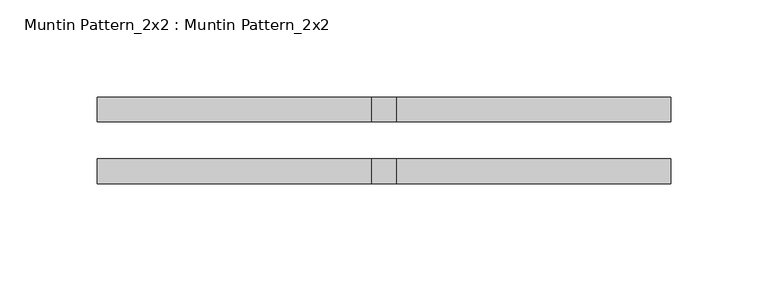
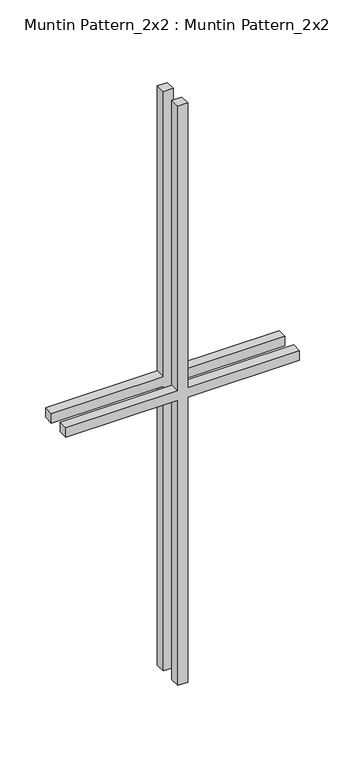
"""IFC4 building model written with IfcOpenShell, lengths in millimetres: proxy geometry, Muntin Pattern_2x2 : Muntin Pattern_2x2."""

from ifc_helpers import new_model, si_unit, frame, origin, place, context, project, spatial, polyline, outline, extrude, source, transform, mapped, element, save


def muntin_pattern_2x2_muntin_pattern_2x2_b3fe6957(model_context):
    return source(origin(), model_context, "Body", "SweptSolid", [
        extrude(outline(polyline([(393.7, -6.35), (393.7, -147.6375), (381.0, -147.6375), (381.0, -6.35), (0.0, -6.35), (0.0, 6.35), (381.0, 6.35), (381.0, 147.6375), (393.7, 147.6375), (393.7, 6.35), (774.7, 6.35), (774.7, -6.35), (393.7, -6.35)])), frame((0.0, 9.525, 0.0), z_axis=(0.0, 1.0, 0.0), x_axis=(0.0, 0.0, 1.0)), (0.0, 0.0, 1.0), 12.7),
        extrude(outline(polyline([(393.7, -6.35), (393.7, -147.6375), (381.0, -147.6375), (381.0, -6.35), (0.0, -6.35), (0.0, 6.35), (381.0, 6.35), (381.0, 147.6375), (393.7, 147.6375), (393.7, 6.35), (774.7, 6.35), (774.7, -6.35), (393.7, -6.35)])), frame((0.0, -22.225, 0.0), z_axis=(0.0, 1.0, 0.0), x_axis=(0.0, 0.0, 1.0)), (0.0, 0.0, 1.0), 12.7),
    ])


if __name__ == "__main__":
    model = new_model("IFC4")
    model_context = context("Model", 3, world=origin())
    ifc_project = project(units=[si_unit("LENGTHUNIT", "METRE", prefix="MILLI")], contexts=[model_context])
    site = spatial("IfcSite", under=ifc_project)
    building = spatial("IfcBuilding", under=site)
    placement = place(None, origin())
    muntin_pattern_2x2_muntin_pattern_2x2_shape = muntin_pattern_2x2_muntin_pattern_2x2_b3fe6957(model_context)
    element("IfcBuildingElementProxy", 1, Name="Muntin Pattern_2x2 : Muntin Pattern_2x2", ObjectType="Muntin Pattern_2x2 : Muntin Pattern_2x2", at=placement, inside=building, context=model_context, shape_type="MappedRepresentation", body=[
        mapped(muntin_pattern_2x2_muntin_pattern_2x2_shape, transform((0.0, 0.0, 0.0), x_axis=(1.0, 0.0, 0.0), y_axis=(0.0, 1.0, 0.0), z_axis=(0.0, 0.0, 1.0))),
    ])
    save(model, "model.ifc")

# Revit data of these elements
# Type "Muntin Pattern_2x2 : Muntin Pattern_2x2"
#   Width [instance default] = 4' - 0"
#   Thickness = 0' - 0 1/2"
#   Height [instance default] = 4' - 0"
#   Distance = 0' - 0 3/4"
#   Interior Material [instance default] = none
#   Exterior Material [instance default] = none
#   Default Elevation = 0
# Element 1 (IfcBuildingElementProxy, "Muntin Pattern_2x2 : Muntin Pattern_2x2")
#   Width = 0' - 11 5/8"
#   Height = 2' - 6 1/2"
#   Interior Material = Wood - Stained
#   Exterior Material = Clad - White
#   Materials on its faces: "Clad - White", "Wood - Stained"
# Materials
#   "Clad - White": class "Wood", colour RGB 242 242 238, transparency 0, Cost = 0
#   "Wood - Stained": class "Wood", colour RGB 224 178 126, transparency 0, Cost = 0
